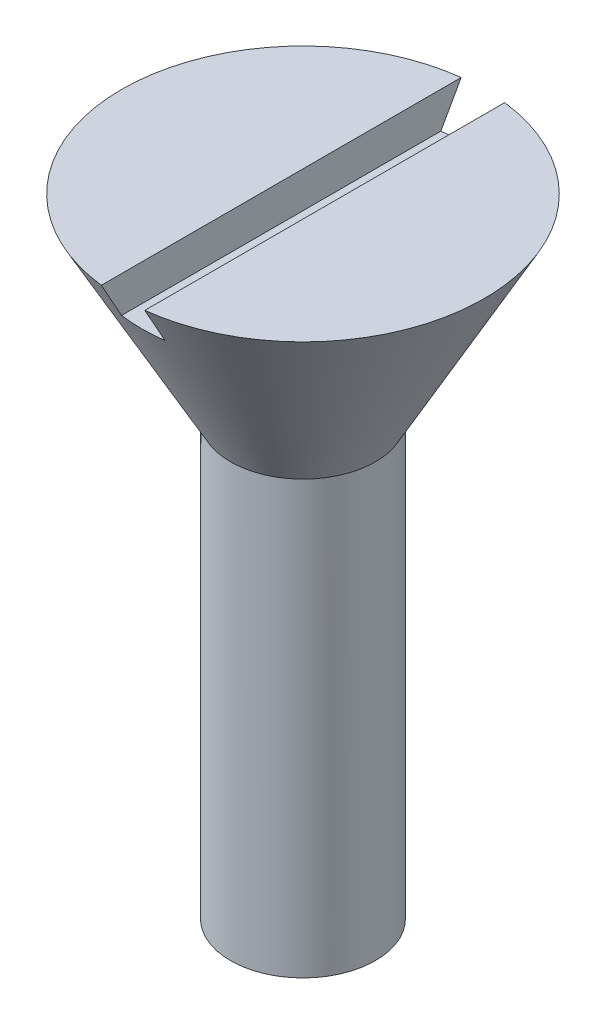
ISO-10303-21;
HEADER;
FILE_DESCRIPTION(('STEP AP214'),'2;1');
FILE_NAME('part.step','',(''),(''),'','','');
FILE_SCHEMA(('AUTOMOTIVE_DESIGN { 1 0 10303 214 1 1 1 1 }'));
ENDSEC;
DATA;
#1=APPLICATION_CONTEXT('core data for automotive mechanical design processes');
#2=APPLICATION_PROTOCOL_DEFINITION('international standard','automotive_design',2000,#1);
#3=PRODUCT_CONTEXT('',#1,'mechanical');
#4=PRODUCT('Part','Part','',(#3));
#5=PRODUCT_RELATED_PRODUCT_CATEGORY('part','',(#4));
#6=PRODUCT_DEFINITION_FORMATION('','',#4);
#7=PRODUCT_DEFINITION_CONTEXT('part definition',#1,'design');
#8=PRODUCT_DEFINITION('design','',#6,#7);
#9=PRODUCT_DEFINITION_SHAPE('','',#8);
#10=(LENGTH_UNIT() NAMED_UNIT(*) SI_UNIT(.MILLI.,.METRE.));
#11=(NAMED_UNIT(*) PLANE_ANGLE_UNIT() SI_UNIT($,.RADIAN.));
#12=(NAMED_UNIT(*) SI_UNIT($,.STERADIAN.) SOLID_ANGLE_UNIT());
#13=UNCERTAINTY_MEASURE_WITH_UNIT(LENGTH_MEASURE(1.E-05),#10,'distance_accuracy_value','');
#14=(GEOMETRIC_REPRESENTATION_CONTEXT(3) GLOBAL_UNCERTAINTY_ASSIGNED_CONTEXT((#13)) GLOBAL_UNIT_ASSIGNED_CONTEXT((#10,
#11,#12)) REPRESENTATION_CONTEXT('',''));
#15=CARTESIAN_POINT('',(0.,0.,0.));
#16=DIRECTION('',(0.,0.,1.));
#17=DIRECTION('',(1.,0.,0.));
#18=AXIS2_PLACEMENT_3D('',#15,#16,#17);
#19=CARTESIAN_POINT('',(0.,68.,0.));
#20=DIRECTION('',(0.,1.,0.));
#21=DIRECTION('',(-1.,0.,0.));
#22=AXIS2_PLACEMENT_3D('',#19,#20,#21);
#23=CYLINDRICAL_SURFACE('',#22,5.);
#24=CARTESIAN_POINT('',(0.,50.,0.));
#25=DIRECTION('',(0.,1.,0.));
#26=DIRECTION('',(-1.,0.,0.));
#27=AXIS2_PLACEMENT_3D('',#24,#25,#26);
#28=CIRCLE('',#27,5.);
#29=CARTESIAN_POINT('',(-4.99999999999999,50.,0.));
#30=VERTEX_POINT('',#29);
#31=EDGE_CURVE('E138',#30,#30,#28,.T.);
#32=ORIENTED_EDGE('',*,*,#31,.F.);
#33=EDGE_LOOP('',(#32));
#34=FACE_BOUND('',#33,.T.);
#35=CARTESIAN_POINT('',(0.,20.204065748598,0.));
#36=DIRECTION('',(0.,-1.,0.));
#37=DIRECTION('',(0.,0.,-1.));
#38=AXIS2_PLACEMENT_3D('',#35,#36,#37);
#39=CIRCLE('',#38,5.);
#40=CARTESIAN_POINT('',(0.,20.204065748598,-5.));
#41=VERTEX_POINT('',#40);
#42=EDGE_CURVE('E45',#41,#41,#39,.T.);
#43=ORIENTED_EDGE('',*,*,#42,.F.);
#44=EDGE_LOOP('',(#43));
#45=FACE_BOUND('',#44,.T.);
#46=ADVANCED_FACE('F39',(#34,#45),#23,.T.);
#47=CARTESIAN_POINT('',(0.,50.,0.));
#48=DIRECTION('',(0.,1.,0.));
#49=DIRECTION('',(-1.,0.,0.));
#50=AXIS2_PLACEMENT_3D('',#47,#48,#49);
#51=CONICAL_SURFACE('',#50,5.,0.507098504392337);
#52=CARTESIAN_POINT('',(1.49999999999998,68.0007,14.9252024045874));
#53=CARTESIAN_POINT('',(1.49999999999998,67.2653661135659,14.5146181085151));
#54=CARTESIAN_POINT('',(1.49999999999999,66.5300982044846,14.1039155460228));
#55=CARTESIAN_POINT('',(1.5,65.0597494174893,13.2821728118846));
#56=CARTESIAN_POINT('',(1.5,64.3246685398994,12.8711326396587));
#57=CARTESIAN_POINT('',(1.50000000000001,62.8546451464812,12.048555552987));
#58=CARTESIAN_POINT('',(1.50000000000001,62.119702666031,11.6370185753054));
#59=CARTESIAN_POINT('',(1.50000000000002,60.6501541837317,10.8133466197689));
#60=CARTESIAN_POINT('',(1.50000000000003,59.9155481814124,10.4012116427525));
#61=CARTESIAN_POINT('',(1.50000000000003,58.4482809616388,9.57692509348955));
#62=CARTESIAN_POINT('',(1.50000000000004,57.7156187965519,9.16477520885056));
#63=CARTESIAN_POINT('',(1.50000000000005,56.2509923505736,8.33922987281977));
#64=CARTESIAN_POINT('',(1.50000000000005,55.5190280726254,7.92583441620537));
#65=CARTESIAN_POINT('',(1.50000000000006,54.0562686349947,7.09716223978929));
#66=CARTESIAN_POINT('',(1.50000000000006,53.3254733566209,6.68188572986674));
#67=CARTESIAN_POINT('',(1.50000000000007,52.2307069396452,6.05647897987081));
#68=CARTESIAN_POINT('',(1.50000000000007,51.866023821464,5.84759546596999));
#69=CARTESIAN_POINT('',(1.50000000000008,51.1373171413246,5.42868154966096));
#70=CARTESIAN_POINT('',(1.50000000000008,50.7732935779261,5.21865114976124));
#71=CARTESIAN_POINT('',(1.50000000000008,50.2178841895837,4.89654250864141));
#72=CARTESIAN_POINT('',(1.50000000000008,50.0261588471004,4.78504975659315));
#73=CARTESIAN_POINT('',(1.50000000000009,49.6430324839687,4.56150705139518));
#74=CARTESIAN_POINT('',(1.50000000000009,49.4516314640999,4.44945709690878));
#75=CARTESIAN_POINT('',(1.50000000000009,49.0691998018953,4.22464700739982));
#76=CARTESIAN_POINT('',(1.50000000000009,48.87816923337,4.11188674674197));
#77=CARTESIAN_POINT('',(1.50000000000009,48.4966257355528,3.88549554753257));
#78=CARTESIAN_POINT('',(1.50000000000009,48.3061128033028,3.77186461397071));
#79=CARTESIAN_POINT('',(1.5000000000001,47.9254095332262,3.54326911694333));
#80=CARTESIAN_POINT('',(1.5000000000001,47.735220439452,3.4283024794168));
#81=CARTESIAN_POINT('',(1.5000000000001,47.3557500313601,3.19688113953137));
#82=CARTESIAN_POINT('',(1.5000000000001,47.166468709533,3.0804264495115));
#83=CARTESIAN_POINT('',(1.5000000000001,46.7892360633675,2.84552809180228));
#84=CARTESIAN_POINT('',(1.5000000000001,46.6012842873916,2.72708515067139));
#85=CARTESIAN_POINT('',(1.50000000000011,46.2272159511182,2.48734217177775));
#86=CARTESIAN_POINT('',(1.50000000000011,46.0410992814868,2.36604230570509));
#87=CARTESIAN_POINT('',(1.50000000000011,45.7210255664681,2.15210395392116));
#88=CARTESIAN_POINT('',(1.50000000000011,45.5864066612115,2.06045769353553));
#89=CARTESIAN_POINT('',(1.50000000000011,45.3193191562247,1.87387804165281));
#90=CARTESIAN_POINT('',(1.50000000000011,45.1868519361409,1.7789426546102));
#91=CARTESIAN_POINT('',(1.50000000000011,44.9908806256576,1.63303763961157));
#92=CARTESIAN_POINT('',(1.50000000000011,44.9260510661643,1.58385051003389));
#93=CARTESIAN_POINT('',(1.50000000000011,44.7975427990405,1.48399860758322));
#94=CARTESIAN_POINT('',(1.50000000000011,44.7338640037927,1.43333394798101));
#95=CARTESIAN_POINT('',(1.50000000000012,44.6080838074975,1.33019604923138));
#96=CARTESIAN_POINT('',(1.50000000000012,44.5459809593111,1.27772458191977));
#97=CARTESIAN_POINT('',(1.50000000000012,44.4238590048742,1.17042092043748));
#98=CARTESIAN_POINT('',(1.50000000000012,44.3638392981725,1.11558941691233));
#99=CARTESIAN_POINT('',(1.50000000000012,44.2660579817322,1.02140817965089));
#100=CARTESIAN_POINT('',(1.50000000000012,44.2274785551411,0.98291011941144));
#101=CARTESIAN_POINT('',(1.50000000000012,44.1520525872863,0.904214678838973));
#102=CARTESIAN_POINT('',(1.50000000000012,44.1152066501561,0.864016715210366));
#103=CARTESIAN_POINT('',(1.50000000000012,44.0439235730426,0.78167398316508));
#104=CARTESIAN_POINT('',(1.50000000000012,44.009481327542,0.739533677627283));
#105=CARTESIAN_POINT('',(1.50000000000012,43.9437950626091,0.652850790206018));
#106=CARTESIAN_POINT('',(1.50000000000012,43.9125486295478,0.60831006064375));
#107=CARTESIAN_POINT('',(1.50000000000012,43.8524951725413,0.513273715285815));
#108=CARTESIAN_POINT('',(1.50000000000012,43.8239962632489,0.462579094045355));
#109=CARTESIAN_POINT('',(1.50000000000012,43.7742375275576,0.357730569081031));
#110=CARTESIAN_POINT('',(1.50000000000012,43.7529656318876,0.303582613959025));
#111=CARTESIAN_POINT('',(1.50000000000012,43.7228735658263,0.201045068976301));
#112=CARTESIAN_POINT('',(1.50000000000012,43.7126224399622,0.153086821182544));
#113=CARTESIAN_POINT('',(1.50000000000012,43.7004926008082,0.0561257785599217));
#114=CARTESIAN_POINT('',(1.50000000000012,43.698605641667,0.00712406036361023));
#115=CARTESIAN_POINT('',(1.50000000000012,43.7034756723007,-0.090425017133062));
#116=CARTESIAN_POINT('',(1.50000000000012,43.7102315505387,-0.138972434051353));
#117=CARTESIAN_POINT('',(1.50000000000012,43.7314167583165,-0.234341217476705));
#118=CARTESIAN_POINT('',(1.50000000000012,43.7458541105535,-0.28116072454547));
#119=CARTESIAN_POINT('',(1.50000000000012,43.7911092991805,-0.399306102383318));
#120=CARTESIAN_POINT('',(1.50000000000012,43.8265668048544,-0.46883264582368));
#121=CARTESIAN_POINT('',(1.50000000000012,43.8869442956127,-0.56863693997851));
#122=CARTESIAN_POINT('',(1.50000000000012,43.9083292908211,-0.601230954393894));
#123=CARTESIAN_POINT('',(1.50000000000012,43.9530199740569,-0.665072019090265));
#124=CARTESIAN_POINT('',(1.50000000000012,43.9763249222429,-0.69631958121371));
#125=CARTESIAN_POINT('',(1.50000000000012,44.0483937071061,-0.788139999577969));
#126=CARTESIAN_POINT('',(1.50000000000012,44.0994050324196,-0.846937398634806));
#127=CARTESIAN_POINT('',(1.50000000000012,44.2053279844848,-0.960937892990754));
#128=CARTESIAN_POINT('',(1.50000000000012,44.2602436455382,-1.0161371541265));
#129=CARTESIAN_POINT('',(1.50000000000012,44.372906442873,-1.12391881259728));
#130=CARTESIAN_POINT('',(1.50000000000012,44.4306621384461,-1.17649219771014));
#131=CARTESIAN_POINT('',(1.50000000000012,44.5480803992412,-1.2794685168499));
#132=CARTESIAN_POINT('',(1.50000000000012,44.6077432999614,-1.32987106530164));
#133=CARTESIAN_POINT('',(1.50000000000011,44.7290410627944,-1.42942327802543));
#134=CARTESIAN_POINT('',(1.50000000000011,44.7906891915874,-1.47855670629244));
#135=CARTESIAN_POINT('',(1.50000000000011,44.9150789190052,-1.57542582703255));
#136=CARTESIAN_POINT('',(1.50000000000011,44.9778206163173,-1.62316139230508));
#137=CARTESIAN_POINT('',(1.50000000000011,45.1040123009586,-1.71738743349821));
#138=CARTESIAN_POINT('',(1.50000000000011,45.1674603981833,-1.76388044713128));
#139=CARTESIAN_POINT('',(1.50000000000011,45.2950290564032,-1.85592650898974));
#140=CARTESIAN_POINT('',(1.50000000000011,45.3591495882952,-1.90147959764416));
#141=CARTESIAN_POINT('',(1.50000000000011,45.5497096516749,-2.03513567192847));
#142=CARTESIAN_POINT('',(1.50000000000011,45.6769229477605,-2.12213512813253));
#143=CARTESIAN_POINT('',(1.50000000000011,45.9327983413799,-2.29398095441287));
#144=CARTESIAN_POINT('',(1.50000000000011,46.0614605274341,-2.37882719189581));
#145=CARTESIAN_POINT('',(1.50000000000011,46.3198630152426,-2.54691391603985));
#146=CARTESIAN_POINT('',(1.5000000000001,46.4496035196755,-2.63015409059474));
#147=CARTESIAN_POINT('',(1.5000000000001,46.7098803297918,-2.7953822311728));
#148=CARTESIAN_POINT('',(1.5000000000001,46.8404166469531,-2.87737017907517));
#149=CARTESIAN_POINT('',(1.5000000000001,47.2332931971782,-3.12209050028796));
#150=CARTESIAN_POINT('',(1.5000000000001,47.4965486780043,-3.28335250022247));
#151=CARTESIAN_POINT('',(1.5000000000001,48.0245674391498,-3.60330890282346));
#152=CARTESIAN_POINT('',(1.50000000000009,48.2893305455806,-3.76200359380466));
#153=CARTESIAN_POINT('',(1.50000000000009,48.817487261848,-4.07617349971999));
#154=CARTESIAN_POINT('',(1.50000000000009,49.0808712628269,-4.231664884094));
#155=CARTESIAN_POINT('',(1.50000000000009,49.6083875354615,-4.54138868356286));
#156=CARTESIAN_POINT('',(1.50000000000008,49.8725198282394,-4.69562106263293));
#157=CARTESIAN_POINT('',(1.50000000000008,50.4011701101299,-5.00304474809423));
#158=CARTESIAN_POINT('',(1.50000000000008,50.6656877585954,-5.15623664064337));
#159=CARTESIAN_POINT('',(1.50000000000008,51.1951413456847,-5.46188978831251));
#160=CARTESIAN_POINT('',(1.50000000000008,51.4600772804293,-5.61435105015616));
#161=CARTESIAN_POINT('',(1.50000000000007,52.3951395915914,-6.15113026056389));
#162=CARTESIAN_POINT('',(1.50000000000007,53.0661330978801,-6.53393722575501));
#163=CARTESIAN_POINT('',(1.50000000000006,54.4093030113565,-7.29747545848057));
#164=CARTESIAN_POINT('',(1.50000000000005,55.0814794257317,-7.67820671334492));
#165=CARTESIAN_POINT('',(1.50000000000005,56.4267736547879,-8.43843026872456));
#166=CARTESIAN_POINT('',(1.50000000000004,57.0998916758482,-8.81792220395369));
#167=CARTESIAN_POINT('',(1.50000000000004,58.4466367804105,-9.57599764717743));
#168=CARTESIAN_POINT('',(1.50000000000003,59.1202638627574,-9.95458115722531));
#169=CARTESIAN_POINT('',(1.50000000000002,60.4775374092657,-10.716525460291));
#170=CARTESIAN_POINT('',(1.50000000000002,61.1611890943176,-11.0998769515799));
#171=CARTESIAN_POINT('',(1.50000000000001,62.5287646726224,-11.8660952271484));
#172=CARTESIAN_POINT('',(1.50000000000001,63.2126885660837,-12.2489620110557));
#173=CARTESIAN_POINT('',(1.5,64.580537893978,-13.0142180816759));
#174=CARTESIAN_POINT('',(1.5,65.2644632681545,-13.3966074761072));
#175=CARTESIAN_POINT('',(1.49999999999999,66.632473117529,-14.1610999929462));
#176=CARTESIAN_POINT('',(1.49999999999998,67.3165575925695,-14.5432031156358));
#177=CARTESIAN_POINT('',(1.49999999999998,68.0007,-14.9252024045874));
#178=B_SPLINE_CURVE_WITH_KNOTS('',3,(#52,#53,#54,#55,#56,#57,#58,#59,#60,#61,#62,#63,#64,#65,
#66,#67,#68,#69,#70,#71,#72,#73,#74,#75,#76,#77,#78,#79,#80,#81,#82,#83,#84,#85,#86,#87,#88,#89,
#90,#91,#92,#93,#94,#95,#96,#97,#98,#99,#100,#101,#102,#103,#104,#105,#106,#107,#108,#109,#110,
#111,#112,#113,#114,#115,#116,#117,#118,#119,#120,#121,#122,#123,#124,#125,#126,#127,#128,#129,
#130,#131,#132,#133,#134,#135,#136,#137,#138,#139,#140,#141,#142,#143,#144,#145,#146,#147,#148,
#149,#150,#151,#152,#153,#154,#155,#156,#157,#158,#159,#160,#161,#162,#163,#164,#165,#166,#167,
#168,#169,#170,#171,#172,#173,#174,#175,#176,#177),.UNSPECIFIED.,.F.,.F.,(4,2,2,2,2,2,2,2,2,2,2,
2,2,2,2,2,2,2,2,2,2,2,2,2,2,2,2,2,2,2,2,2,2,2,2,2,2,2,2,2,2,2,2,2,2,2,2,2,2,2,2,2,2,2,2,2,2,2,2,
2,2,2,4),(0.,2.52659035590981,5.05318506049076,7.58014511927942,10.1071016375379,
12.6289953313502,15.1508996140235,17.6725291243828,18.9333350759924,20.1941382710398,
20.8594969863601,21.5248572986164,22.1903387998612,22.8558164901898,23.5225222171262,
24.1892224192737,24.8556840781416,25.5221057869393,26.0106396408097,26.4994752701318,
26.7435910257797,26.9876881159077,27.2315522938255,27.4753455857244,27.6388107988615,
27.802332565067,27.9654957115597,28.1285347051498,28.3026054537262,28.4763840547136,
28.6228684074507,28.7692083157679,28.9155294055134,29.0620036170163,29.2947076523754,
29.4116277743003,29.5285030506908,29.7617341343803,29.9952098171251,30.2294383591756,
30.4637083338111,30.7001810130547,30.9366751440241,31.1726422258755,31.4085991368185,
31.8709154054895,32.3332600744554,32.7956937038761,33.258134018779,34.184271683259,
35.1103046080594,36.0278714969102,36.9454645493377,37.8624887158918,38.7795044272191,
41.0970298300953,43.414569363304,45.7327394636736,48.0509043194229,50.402295532897,
52.7536885514041,55.1043862659194,57.4550816624755),.UNSPECIFIED.);
#179=CARTESIAN_POINT('',(1.50000000000002,61.,-11.0093955385142));
#180=VERTEX_POINT('',#179);
#181=CARTESIAN_POINT('',(1.50000000000001,63.5016844532272,-12.4106162642895));
#182=VERTEX_POINT('',#181);
#183=EDGE_CURVE('E90',#180,#182,#178,.T.);
#184=ORIENTED_EDGE('',*,*,#183,.T.);
#185=CARTESIAN_POINT('',(0.,63.5016844532272,0.));
#186=DIRECTION('',(0.,-1.,0.));
#187=DIRECTION('',(0.,0.,-1.));
#188=AXIS2_PLACEMENT_3D('',#185,#186,#187);
#189=CIRCLE('',#188,12.5009358073485);
#190=CARTESIAN_POINT('',(1.50000000000001,63.5016844532272,12.4106162642895));
#191=VERTEX_POINT('',#190);
#192=EDGE_CURVE('E58',#182,#191,#189,.T.);
#193=ORIENTED_EDGE('',*,*,#192,.T.);
#194=CARTESIAN_POINT('',(1.50000000000002,61.,11.0093955385142));
#195=VERTEX_POINT('',#194);
#196=EDGE_CURVE('E81',#191,#195,#178,.T.);
#197=ORIENTED_EDGE('',*,*,#196,.T.);
#198=CARTESIAN_POINT('',(0.,61.,0.));
#199=DIRECTION('',(0.,-1.,0.));
#200=DIRECTION('',(0.,0.,-1.));
#201=AXIS2_PLACEMENT_3D('',#198,#199,#200);
#202=CIRCLE('',#201,11.1111111111111);
#203=CARTESIAN_POINT('',(-1.49999999999998,61.,11.0093955385142));
#204=VERTEX_POINT('',#203);
#205=EDGE_CURVE('E50',#195,#204,#202,.T.);
#206=ORIENTED_EDGE('',*,*,#205,.T.);
#207=CARTESIAN_POINT('',(-1.49999999999998,68.0007,-14.9252024045874));
#208=CARTESIAN_POINT('',(-1.49999999999998,67.2653661135659,-14.5146181085151));
#209=CARTESIAN_POINT('',(-1.49999999999998,66.5300982044846,-14.1039155460228));
#210=CARTESIAN_POINT('',(-1.49999999999998,65.0597494174893,-13.2821728118845));
#211=CARTESIAN_POINT('',(-1.49999999999998,64.3246685398994,-12.8711326396587));
#212=CARTESIAN_POINT('',(-1.49999999999998,62.8546451464811,-12.048555552987));
#213=CARTESIAN_POINT('',(-1.49999999999998,62.1197026660309,-11.6370185753054));
#214=CARTESIAN_POINT('',(-1.49999999999998,60.6501541837316,-10.8133466197688));
#215=CARTESIAN_POINT('',(-1.49999999999998,59.9155481814123,-10.4012116427525));
#216=CARTESIAN_POINT('',(-1.49999999999998,58.4482809616387,-9.57692509348948));
#217=CARTESIAN_POINT('',(-1.49999999999998,57.7156187965518,-9.16477520885051));
#218=CARTESIAN_POINT('',(-1.49999999999998,56.2509923505735,-8.33922987281973));
#219=CARTESIAN_POINT('',(-1.49999999999998,55.5190280726253,-7.92583441620534));
#220=CARTESIAN_POINT('',(-1.49999999999998,54.0562686349946,-7.09716223978926));
#221=CARTESIAN_POINT('',(-1.49999999999998,53.3254733566209,-6.68188572986672));
#222=CARTESIAN_POINT('',(-1.49999999999998,52.2307069396452,-6.05647897987081));
#223=CARTESIAN_POINT('',(-1.49999999999998,51.866023821464,-5.84759546597));
#224=CARTESIAN_POINT('',(-1.49999999999998,51.1373171413246,-5.42868154966097));
#225=CARTESIAN_POINT('',(-1.49999999999998,50.7732935779261,-5.21865114976126));
#226=CARTESIAN_POINT('',(-1.49999999999998,50.2178841895837,-4.89654250864143));
#227=CARTESIAN_POINT('',(-1.49999999999998,50.0261588471004,-4.78504975659317));
#228=CARTESIAN_POINT('',(-1.49999999999998,49.6430324839687,-4.56150705139521));
#229=CARTESIAN_POINT('',(-1.49999999999998,49.4516314640998,-4.44945709690881));
#230=CARTESIAN_POINT('',(-1.49999999999998,49.0691998018953,-4.22464700739985));
#231=CARTESIAN_POINT('',(-1.49999999999998,48.87816923337,-4.111886746742));
#232=CARTESIAN_POINT('',(-1.49999999999998,48.4966257355528,-3.88549554753261));
#233=CARTESIAN_POINT('',(-1.49999999999998,48.3061128033028,-3.77186461397075));
#234=CARTESIAN_POINT('',(-1.49999999999998,47.9254095332262,-3.54326911694337));
#235=CARTESIAN_POINT('',(-1.49999999999998,47.735220439452,-3.42830247941684));
#236=CARTESIAN_POINT('',(-1.49999999999998,47.3557500313601,-3.19688113953141));
#237=CARTESIAN_POINT('',(-1.49999999999998,47.166468709533,-3.08042644951155));
#238=CARTESIAN_POINT('',(-1.49999999999998,46.7892360633675,-2.84552809180233));
#239=CARTESIAN_POINT('',(-1.49999999999998,46.6012842873916,-2.72708515067144));
#240=CARTESIAN_POINT('',(-1.49999999999998,46.2272159511182,-2.48734217177781));
#241=CARTESIAN_POINT('',(-1.49999999999998,46.0410992814867,-2.36604230570515));
#242=CARTESIAN_POINT('',(-1.49999999999998,45.721025566468,-2.15210395392119));
#243=CARTESIAN_POINT('',(-1.49999999999998,45.5864066612114,-2.06045769353554));
#244=CARTESIAN_POINT('',(-1.49999999999998,45.3193191562245,-1.87387804165276));
#245=CARTESIAN_POINT('',(-1.49999999999998,45.1868519361406,-1.77894265461013));
#246=CARTESIAN_POINT('',(-1.49999999999998,44.9908806256573,-1.63303763961145));
#247=CARTESIAN_POINT('',(-1.49999999999998,44.926051066164,-1.58385051003375));
#248=CARTESIAN_POINT('',(-1.49999999999998,44.7975427990401,-1.48399860758305));
#249=CARTESIAN_POINT('',(-1.49999999999998,44.7338640037923,-1.43333394798083));
#250=CARTESIAN_POINT('',(-1.49999999999998,44.6080838074971,-1.33019604923117));
#251=CARTESIAN_POINT('',(-1.49999999999998,44.5459809593106,-1.27772458191954));
#252=CARTESIAN_POINT('',(-1.49999999999998,44.4238590048737,-1.17042092043721));
#253=CARTESIAN_POINT('',(-1.49999999999998,44.363839298172,-1.11558941691204));
#254=CARTESIAN_POINT('',(-1.49999999999998,44.2660579817317,-1.02140817965062));
#255=CARTESIAN_POINT('',(-1.49999999999998,44.2274785551407,-0.982910119411209));
#256=CARTESIAN_POINT('',(-1.49999999999998,44.152052587286,-0.904214678838818));
#257=CARTESIAN_POINT('',(-1.49999999999998,44.1152066501558,-0.864016715210248));
#258=CARTESIAN_POINT('',(-1.49999999999998,44.0439235730424,-0.78167398316504));
#259=CARTESIAN_POINT('',(-1.49999999999998,44.0094813275418,-0.739533677627283));
#260=CARTESIAN_POINT('',(-1.49999999999998,43.943795062609,-0.652850790206106));
#261=CARTESIAN_POINT('',(-1.49999999999998,43.9125486295477,-0.608310060643886));
#262=CARTESIAN_POINT('',(-1.49999999999998,43.8524951725412,-0.513273715285989));
#263=CARTESIAN_POINT('',(-1.49999999999998,43.8239962632488,-0.462579094045515));
#264=CARTESIAN_POINT('',(-1.49999999999998,43.7742375275574,-0.357730569081162));
#265=CARTESIAN_POINT('',(-1.49999999999998,43.7529656318874,-0.303582613959143));
#266=CARTESIAN_POINT('',(-1.49999999999998,43.7228735658261,-0.201045068976406));
#267=CARTESIAN_POINT('',(-1.49999999999998,43.712622439962,-0.153086821182653));
#268=CARTESIAN_POINT('',(-1.49999999999998,43.7004926008079,-0.0561257785600382));
#269=CARTESIAN_POINT('',(-1.49999999999998,43.6986056416668,-0.00712406036373147));
#270=CARTESIAN_POINT('',(-1.49999999999998,43.7034756723005,0.0904250171329353));
#271=CARTESIAN_POINT('',(-1.49999999999998,43.7102315505384,0.138972434051225));
#272=CARTESIAN_POINT('',(-1.49999999999998,43.7314167583162,0.234341217476575));
#273=CARTESIAN_POINT('',(-1.49999999999998,43.7458541105533,0.281160724545338));
#274=CARTESIAN_POINT('',(-1.49999999999998,43.7911092991802,0.399306102383165));
#275=CARTESIAN_POINT('',(-1.49999999999998,43.8265668048541,0.468832645823514));
#276=CARTESIAN_POINT('',(-1.49999999999998,43.8869442956123,0.568636939978319));
#277=CARTESIAN_POINT('',(-1.49999999999998,43.9083292908207,0.601230954393696));
#278=CARTESIAN_POINT('',(-1.49999999999998,43.9530199740565,0.665072019090052));
#279=CARTESIAN_POINT('',(-1.49999999999998,43.9763249222425,0.696319581213489));
#280=CARTESIAN_POINT('',(-1.49999999999998,44.0483937071057,0.78813999957771));
#281=CARTESIAN_POINT('',(-1.49999999999998,44.0994050324192,0.846937398634517));
#282=CARTESIAN_POINT('',(-1.49999999999998,44.2053279844843,0.960937892990408));
#283=CARTESIAN_POINT('',(-1.49999999999998,44.2602436455377,1.01613715412612));
#284=CARTESIAN_POINT('',(-1.49999999999998,44.3729064428723,1.12391881259685));
#285=CARTESIAN_POINT('',(-1.49999999999998,44.4306621384454,1.17649219770969));
#286=CARTESIAN_POINT('',(-1.49999999999998,44.5480803992404,1.2794685168494));
#287=CARTESIAN_POINT('',(-1.49999999999998,44.6077432999606,1.32987106530111));
#288=CARTESIAN_POINT('',(-1.49999999999998,44.7290410627935,1.42942327802485));
#289=CARTESIAN_POINT('',(-1.49999999999998,44.7906891915864,1.47855670629184));
#290=CARTESIAN_POINT('',(-1.49999999999998,44.9150789190041,1.5754258270319));
#291=CARTESIAN_POINT('',(-1.49999999999998,44.9778206163162,1.6231613923044));
#292=CARTESIAN_POINT('',(-1.49999999999998,45.1040123009575,1.71738743349748));
#293=CARTESIAN_POINT('',(-1.49999999999998,45.1674603981821,1.76388044713053));
#294=CARTESIAN_POINT('',(-1.49999999999998,45.2950290564019,1.85592650898895));
#295=CARTESIAN_POINT('',(-1.49999999999998,45.3591495882939,1.90147959764335));
#296=CARTESIAN_POINT('',(-1.49999999999998,45.5497096516735,2.03513567192759));
#297=CARTESIAN_POINT('',(-1.49999999999998,45.676922947759,2.1221351281316));
#298=CARTESIAN_POINT('',(-1.49999999999998,45.9327983413783,2.29398095441185));
#299=CARTESIAN_POINT('',(-1.49999999999998,46.0614605274324,2.37882719189475));
#300=CARTESIAN_POINT('',(-1.49999999999998,46.3198630152407,2.54691391603869));
#301=CARTESIAN_POINT('',(-1.49999999999998,46.4496035196735,2.63015409059354));
#302=CARTESIAN_POINT('',(-1.49999999999998,46.7098803297896,2.79538223117151));
#303=CARTESIAN_POINT('',(-1.49999999999998,46.8404166469509,2.87737017907384));
#304=CARTESIAN_POINT('',(-1.49999999999998,47.2332931971758,3.12209050028649));
#305=CARTESIAN_POINT('',(-1.49999999999998,47.4965486780017,3.28335250022091));
#306=CARTESIAN_POINT('',(-1.49999999999998,48.0245674391468,3.60330890282173));
#307=CARTESIAN_POINT('',(-1.49999999999998,48.2893305455774,3.76200359380284));
#308=CARTESIAN_POINT('',(-1.49999999999998,48.8174872618445,4.07617349971799));
#309=CARTESIAN_POINT('',(-1.49999999999998,49.0808712628233,4.23166488409193));
#310=CARTESIAN_POINT('',(-1.49999999999998,49.6083875354576,4.54138868356062));
#311=CARTESIAN_POINT('',(-1.49999999999998,49.8725198282353,4.6956210626306));
#312=CARTESIAN_POINT('',(-1.49999999999998,50.4011701101255,5.00304474809172));
#313=CARTESIAN_POINT('',(-1.49999999999998,50.6656877585908,5.15623664064078));
#314=CARTESIAN_POINT('',(-1.49999999999998,51.1951413456798,5.46188978830973));
#315=CARTESIAN_POINT('',(-1.49999999999998,51.4600772804243,5.61435105015329));
#316=CARTESIAN_POINT('',(-1.49999999999998,52.3951395915864,6.15113026056107));
#317=CARTESIAN_POINT('',(-1.49999999999998,53.0661330978753,6.53393722575231));
#318=CARTESIAN_POINT('',(-1.49999999999998,54.4093030113522,7.29747545847812));
#319=CARTESIAN_POINT('',(-1.49999999999998,55.0814794257276,7.67820671334259));
#320=CARTESIAN_POINT('',(-1.49999999999998,56.4267736547841,8.43843026872248));
#321=CARTESIAN_POINT('',(-1.49999999999998,57.0998916758447,8.81792220395173));
#322=CARTESIAN_POINT('',(-1.49999999999998,58.4466367804075,9.57599764717571));
#323=CARTESIAN_POINT('',(-1.49999999999998,59.1202638627545,9.95458115722371));
#324=CARTESIAN_POINT('',(-1.49999999999998,60.4775374092633,10.7165254602896));
#325=CARTESIAN_POINT('',(-1.49999999999998,61.1611890943154,11.0998769515787));
#326=CARTESIAN_POINT('',(-1.49999999999998,62.5287646726206,11.8660952271474));
#327=CARTESIAN_POINT('',(-1.49999999999998,63.2126885660822,12.2489620110548));
#328=CARTESIAN_POINT('',(-1.49999999999998,64.5805378939769,13.0142180816753));
#329=CARTESIAN_POINT('',(-1.49999999999998,65.2644632681536,13.3966074761067));
#330=CARTESIAN_POINT('',(-1.49999999999998,66.6324731175285,14.1610999929459));
#331=CARTESIAN_POINT('',(-1.49999999999998,67.3165575925693,14.5432031156357));
#332=CARTESIAN_POINT('',(-1.49999999999998,68.0007,14.9252024045874));
#333=B_SPLINE_CURVE_WITH_KNOTS('',3,(#207,#208,#209,#210,#211,#212,#213,#214,#215,#216,#217,
#218,#219,#220,#221,#222,#223,#224,#225,#226,#227,#228,#229,#230,#231,#232,#233,#234,#235,#236,
#237,#238,#239,#240,#241,#242,#243,#244,#245,#246,#247,#248,#249,#250,#251,#252,#253,#254,#255,
#256,#257,#258,#259,#260,#261,#262,#263,#264,#265,#266,#267,#268,#269,#270,#271,#272,#273,#274,
#275,#276,#277,#278,#279,#280,#281,#282,#283,#284,#285,#286,#287,#288,#289,#290,#291,#292,#293,
#294,#295,#296,#297,#298,#299,#300,#301,#302,#303,#304,#305,#306,#307,#308,#309,#310,#311,#312,
#313,#314,#315,#316,#317,#318,#319,#320,#321,#322,#323,#324,#325,#326,#327,#328,#329,#330,#331,
#332),.UNSPECIFIED.,.F.,.F.,(4,2,2,2,2,2,2,2,2,2,2,2,2,2,2,2,2,2,2,2,2,2,2,2,2,2,2,2,2,2,2,2,2,
2,2,2,2,2,2,2,2,2,2,2,2,2,2,2,2,2,2,2,2,2,2,2,2,2,2,2,2,2,4),(0.,2.52659035590984,
5.05318506049084,7.58014511927955,10.1071016375381,12.6289953313503,15.1508996140236,
17.6725291243829,18.9333350759924,20.1941382710398,20.8594969863601,21.5248572986164,
22.1903387998612,22.8558164901898,23.5225222171262,24.1892224192737,24.8556840781416,
25.5221057869393,26.0106396408099,26.4994752701322,26.74359102578,26.9876881159082,
27.231552293826,27.475345585725,27.6388107988619,27.8023325650673,27.9654957115598,
28.1285347051497,28.3026054537262,28.4763840547136,28.6228684074508,28.7692083157679,
28.9155294055135,29.0620036170164,29.2947076523754,29.4116277743003,29.5285030506907,
29.7617341343801,29.9952098171247,30.2294383591751,30.4637083338105,30.7001810130539,
30.9366751440232,31.1726422258745,31.4085991368173,31.870915405488,32.3332600744537,
32.7956937038741,33.2581340187767,34.1842716832561,35.110304608056,36.0278714969063,
36.9454645493333,37.8624887158867,38.7795044272135,41.0970298300904,43.4145693632999,
45.7327394636702,48.0509043194203,50.4022955328951,52.7536885514029,55.104386265919,
57.4550816624758),.UNSPECIFIED.);
#334=CARTESIAN_POINT('',(-1.49999999999998,63.5016844532272,12.4106162642895));
#335=VERTEX_POINT('',#334);
#336=EDGE_CURVE('E91',#204,#335,#333,.T.);
#337=ORIENTED_EDGE('',*,*,#336,.T.);
#338=CARTESIAN_POINT('',(-1.49999999999998,63.5016844532272,-12.4106162642895));
#339=VERTEX_POINT('',#338);
#340=EDGE_CURVE('E52',#335,#339,#189,.T.);
#341=ORIENTED_EDGE('',*,*,#340,.T.);
#342=CARTESIAN_POINT('',(-1.49999999999998,61.,-11.0093955385142));
#343=VERTEX_POINT('',#342);
#344=EDGE_CURVE('E97',#339,#343,#333,.T.);
#345=ORIENTED_EDGE('',*,*,#344,.T.);
#346=EDGE_CURVE('E152',#343,#180,#202,.T.);
#347=ORIENTED_EDGE('',*,*,#346,.T.);
#348=EDGE_LOOP('',(#184,#193,#197,#206,#337,#341,#345,#347));
#349=FACE_BOUND('',#348,.T.);
#350=ORIENTED_EDGE('',*,*,#31,.T.);
#351=EDGE_LOOP('',(#350));
#352=FACE_BOUND('',#351,.T.);
#353=ADVANCED_FACE('F82',(#349,#352),#51,.T.);
#354=CARTESIAN_POINT('',(-1.49999999999998,61.,-15.));
#355=DIRECTION('',(0.,-1.,0.));
#356=DIRECTION('',(0.,0.,-1.));
#357=AXIS2_PLACEMENT_3D('',#354,#355,#356);
#358=PLANE('',#357);
#359=DIRECTION('',(0.,0.,1.));
#360=VECTOR('',#359,1.);
#361=CARTESIAN_POINT('',(1.50000000000002,61.,-15.));
#362=LINE('',#361,#360);
#363=EDGE_CURVE('E95',#180,#195,#362,.T.);
#364=ORIENTED_EDGE('',*,*,#363,.F.);
#365=ORIENTED_EDGE('',*,*,#346,.F.);
#366=DIRECTION('',(0.,0.,1.));
#367=VECTOR('',#366,1.);
#368=CARTESIAN_POINT('',(-1.49999999999998,61.,-15.));
#369=LINE('',#368,#367);
#370=EDGE_CURVE('E102',#343,#204,#369,.T.);
#371=ORIENTED_EDGE('',*,*,#370,.T.);
#372=ORIENTED_EDGE('',*,*,#205,.F.);
#373=EDGE_LOOP('',(#364,#365,#371,#372));
#374=FACE_BOUND('',#373,.T.);
#375=ADVANCED_FACE('F122',(#374),#358,.F.);
#376=CARTESIAN_POINT('',(-1.49999999999998,68.,-15.));
#377=DIRECTION('',(-1.,0.,0.));
#378=DIRECTION('',(0.,-1.,0.));
#379=AXIS2_PLACEMENT_3D('',#376,#377,#378);
#380=PLANE('',#379);
#381=ORIENTED_EDGE('',*,*,#344,.F.);
#382=DIRECTION('',(0.,0.,1.));
#383=VECTOR('',#382,1.);
#384=CARTESIAN_POINT('',(-1.49999999999998,63.5016844532272,-15.));
#385=LINE('',#384,#383);
#386=EDGE_CURVE('E88',#339,#335,#385,.T.);
#387=ORIENTED_EDGE('',*,*,#386,.T.);
#388=ORIENTED_EDGE('',*,*,#336,.F.);
#389=ORIENTED_EDGE('',*,*,#370,.F.);
#390=EDGE_LOOP('',(#381,#387,#388,#389));
#391=FACE_BOUND('',#390,.T.);
#392=ADVANCED_FACE('F117',(#391),#380,.F.);
#393=CARTESIAN_POINT('',(1.49999999999998,68.,-15.));
#394=DIRECTION('',(1.,0.,0.));
#395=DIRECTION('',(0.,1.,0.));
#396=AXIS2_PLACEMENT_3D('',#393,#394,#395);
#397=PLANE('',#396);
#398=ORIENTED_EDGE('',*,*,#196,.F.);
#399=DIRECTION('',(0.,0.,-1.));
#400=VECTOR('',#399,1.);
#401=CARTESIAN_POINT('',(1.50000000000001,63.5016844532272,-15.));
#402=LINE('',#401,#400);
#403=EDGE_CURVE('E11',#191,#182,#402,.T.);
#404=ORIENTED_EDGE('',*,*,#403,.T.);
#405=ORIENTED_EDGE('',*,*,#183,.F.);
#406=ORIENTED_EDGE('',*,*,#363,.T.);
#407=EDGE_LOOP('',(#398,#404,#405,#406));
#408=FACE_BOUND('',#407,.T.);
#409=ADVANCED_FACE('F92',(#408),#397,.F.);
#410=CARTESIAN_POINT('',(-15.,63.5016844532272,-14.9248115565993));
#411=DIRECTION('',(0.,-1.,0.));
#412=DIRECTION('',(0.,0.,-1.));
#413=AXIS2_PLACEMENT_3D('',#410,#411,#412);
#414=PLANE('',#413);
#415=ORIENTED_EDGE('',*,*,#403,.F.);
#416=ORIENTED_EDGE('',*,*,#192,.F.);
#417=EDGE_LOOP('',(#415,#416));
#418=FACE_BOUND('',#417,.T.);
#419=ADVANCED_FACE('F77',(#418),#414,.F.);
#420=ORIENTED_EDGE('',*,*,#386,.F.);
#421=ORIENTED_EDGE('',*,*,#340,.F.);
#422=EDGE_LOOP('',(#420,#421));
#423=FACE_BOUND('',#422,.T.);
#424=ADVANCED_FACE('F118',(#423),#414,.F.);
#425=CARTESIAN_POINT('',(-18.1656399821502,20.204065748598,12.4106162642895));
#426=DIRECTION('',(0.,-1.,0.));
#427=DIRECTION('',(0.,0.,-1.));
#428=AXIS2_PLACEMENT_3D('',#425,#426,#427);
#429=PLANE('',#428);
#430=ORIENTED_EDGE('',*,*,#42,.T.);
#431=EDGE_LOOP('',(#430));
#432=FACE_BOUND('',#431,.T.);
#433=ADVANCED_FACE('F144',(#432),#429,.T.);
#434=CLOSED_SHELL('',(#46,#353,#375,#392,#409,#419,#424,#433));
#435=MANIFOLD_SOLID_BREP('B2',#434);
#436=ADVANCED_BREP_SHAPE_REPRESENTATION('',(#18,#435),#14);
#437=SHAPE_DEFINITION_REPRESENTATION(#9,#436);
ENDSEC;
END-ISO-10303-21;
